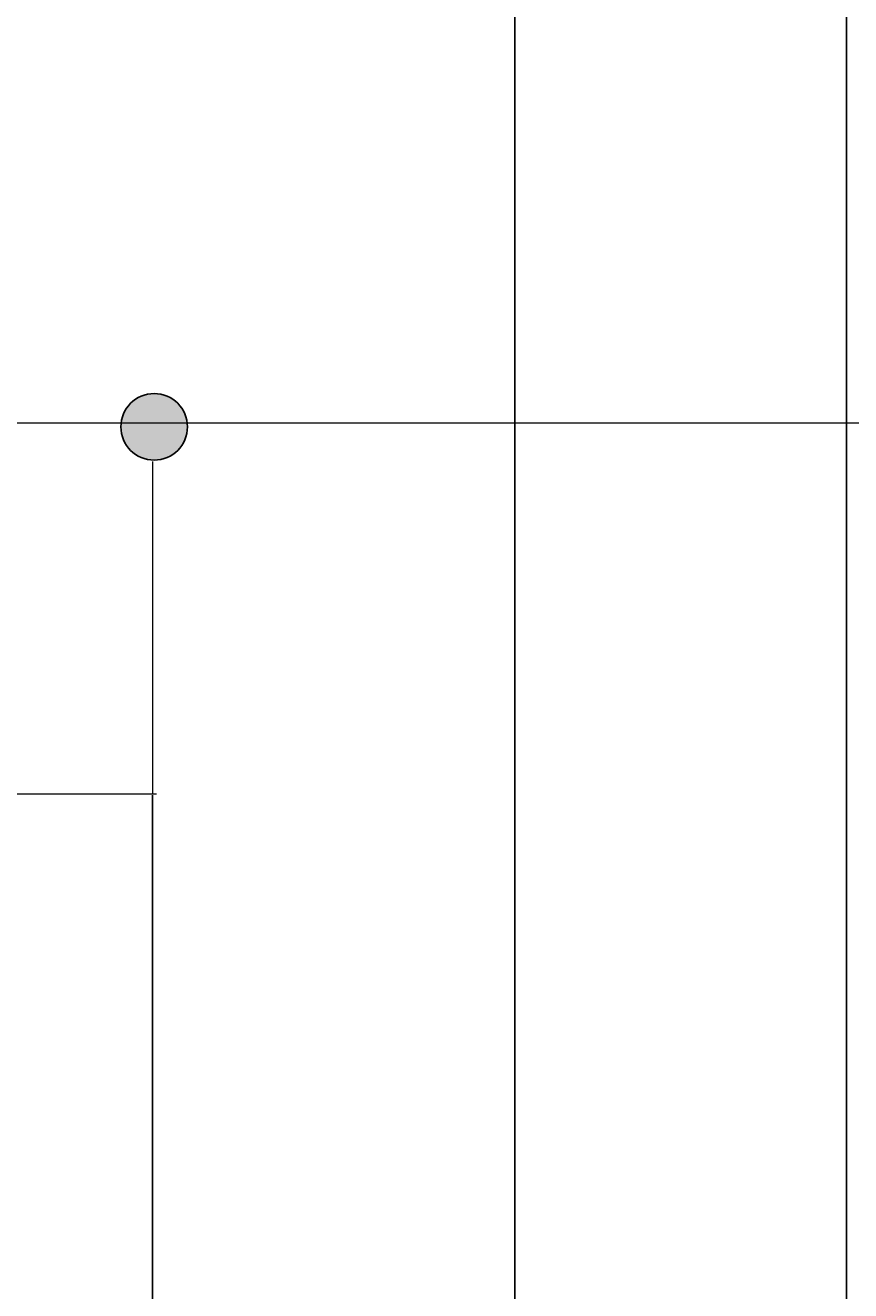
# Model space of a CAD drawing. Units: inches. Extents: x 738 to 1068, y 378 to 757.
# Tile 29 of 41: x 901 to 939, y 492 to 549. Entities that reach past the tile are written whole.
import ezdxf

# ---------------------------------------------------------------- set-up
doc = ezdxf.new("R2010")
doc.units = ezdxf.units.IN
doc.header["$MEASUREMENT"] = 0
for name, color, linetype, lineweight in [('A-ANNO-DIMS', 2, 'Continuous', 18), ('E-CONN', 7, 'Continuous', 25), ('E-CONN-PATT', 7, 'Continuous', 13), ('E-CTRL-WIRE', 7, 'Continuous', 18)]:
    doc.layers.add(name, color=color, linetype=linetype, lineweight=lineweight)
doc.styles.get("Standard").update_dxf_attribs({"font": 'arial.ttf'})
doc.dimstyles.get("Standard").update_dxf_attribs({"dimtxt": 0.18, "dimasz": 0.18, "dimexe": 0.18, "dimexo": 0.0625, "dimgap": 0.09, "dimtad": 0, "dimtih": 1, "dimtoh": 1, "dimdec": 4, "dimzin": 0, "dimdsep": 46, "dimtxsty": 'Standard', "dimcen": 0.09, "dimadec": 0, "dimazin": 0, "dimtfac": 1, "dimtdec": 4, "dimtofl": 0, "dimtmove": 0, "dimatfit": 3, "dimfxl": 1, "dimtolj": 1, "dimtzin": 0, "dimarcsym": 0})

# ---------------------------------------------------------------- blocks, each defined once
blk = doc.blocks.new('*D18')
at = {"layer": 'A-ANNO-DIMS', "color": 0, "lineweight": -2, "transparency": 16777216}
for p, q in [((901.525, 738.375), (1068.179, 738.375)), ((1067.999, 738.195), (1067.999, 569.167)), ((1067.999, 399.775), (1067.999, 568.803)), ((1023.842, 399.595), (1068.179, 399.595))]:
    blk.add_line(p, q, dxfattribs=at)
at = {"layer": 'A-ANNO-DIMS', "color": 0, "transparency": 16777216}
for points in [[(1067.969, 738.195), (1068.029, 738.195), (1067.999, 738.375)], [(1067.969, 399.775), (1068.029, 399.775), (1067.999, 399.595)]]:
    blk.add_solid(points, dxfattribs=at)
at = {"layer": 'Defpoints', "color": 0, "transparency": 16777216}
for p in [(901.462, 738.375), (1067.999, 738.375), (1023.779, 399.595)]:
    blk.add_point(p, dxfattribs=at)
at = {"layer": 'A-ANNO-DIMS', "color": 0, "transparency": 16777216, "insert": (1067.999, 568.985), "char_height": 0.18, "attachment_point": 5}
blk.add_mtext('\\A1;338.8', dxfattribs=at)
blk = doc.blocks.new('*D27')
at = {"layer": 'A-ANNO-DIMS', "color": 0, "lineweight": -2, "transparency": 16777216}
for p, q in [((883.457, 646.923), (883.457, 378.239)), ((923.511, 646.923), (923.511, 378.239)), ((883.637, 378.419), (903.086, 378.419)), ((923.331, 378.419), (903.882, 378.419))]:
    blk.add_line(p, q, dxfattribs=at)
at = {"layer": 'A-ANNO-DIMS', "color": 0, "transparency": 16777216}
for points in [[(883.637, 378.449), (883.637, 378.389), (883.457, 378.419)], [(923.331, 378.449), (923.331, 378.389), (923.511, 378.419)]]:
    blk.add_solid(points, dxfattribs=at)
at = {"layer": 'Defpoints', "color": 0, "transparency": 16777216}
for p in [(883.457, 646.985), (923.511, 646.985), (923.511, 378.419)]:
    blk.add_point(p, dxfattribs=at)
at = {"layer": 'A-ANNO-DIMS', "color": 0, "transparency": 16777216, "insert": (903.484, 378.419), "char_height": 0.18, "attachment_point": 5}
blk.add_mtext('\\A1;40.05', dxfattribs=at)
blk = doc.blocks.new('*D28')
at = {"layer": 'A-ANNO-DIMS', "color": 0, "lineweight": -2, "transparency": 16777216}
for p, q in [((923.511, 646.923), (923.511, 378.239)), ((969.439, 646.923), (969.439, 378.239)), ((923.691, 378.419), (946.078, 378.419)), ((969.259, 378.419), (946.872, 378.419))]:
    blk.add_line(p, q, dxfattribs=at)
at = {"layer": 'A-ANNO-DIMS', "color": 0, "transparency": 16777216}
for points in [[(923.691, 378.449), (923.691, 378.389), (923.511, 378.419)], [(969.259, 378.449), (969.259, 378.389), (969.439, 378.419)]]:
    blk.add_solid(points, dxfattribs=at)
at = {"layer": 'Defpoints', "color": 0, "transparency": 16777216}
for p in [(923.511, 646.985), (969.439, 646.985), (969.439, 378.419)]:
    blk.add_point(p, dxfattribs=at)
at = {"layer": 'A-ANNO-DIMS', "color": 0, "transparency": 16777216, "insert": (946.475, 378.419), "char_height": 0.18, "attachment_point": 5}
blk.add_mtext('\\A1;45.93', dxfattribs=at)
blk = doc.blocks.new('*D33')
at = {"layer": 'A-ANNO-DIMS', "color": 0, "lineweight": -2, "transparency": 16777216}
for p, q in [((836.324, 514.624), (836.324, 378.239)), ((907.171, 514.624), (907.171, 378.239)), ((836.504, 378.419), (871.354, 378.419)), ((906.991, 378.419), (872.141, 378.419))]:
    blk.add_line(p, q, dxfattribs=at)
at = {"layer": 'A-ANNO-DIMS', "color": 0, "transparency": 16777216}
for points in [[(836.504, 378.449), (836.504, 378.389), (836.324, 378.419)], [(906.991, 378.449), (906.991, 378.389), (907.171, 378.419)]]:
    blk.add_solid(points, dxfattribs=at)
at = {"layer": 'Defpoints', "color": 0, "transparency": 16777216}
for p in [(836.324, 514.687), (907.171, 514.687), (907.171, 378.419)]:
    blk.add_point(p, dxfattribs=at)
at = {"layer": 'A-ANNO-DIMS', "color": 0, "transparency": 16777216, "insert": (871.748, 378.419), "char_height": 0.18, "attachment_point": 5}
blk.add_mtext('\\A1;70.85', dxfattribs=at)
blk = doc.blocks.new('*D39')
at = {"layer": 'A-ANNO-DIMS', "color": 0, "lineweight": -2, "transparency": 16777216}
for p, q in [((887.04, 581.418), (887.04, 378.239)), ((938.455, 581.418), (938.455, 378.239)), ((887.22, 378.419), (912.371, 378.419)), ((938.275, 378.419), (913.124, 378.419))]:
    blk.add_line(p, q, dxfattribs=at)
at = {"layer": 'A-ANNO-DIMS', "color": 0, "transparency": 16777216}
for points in [[(887.22, 378.449), (887.22, 378.389), (887.04, 378.419)], [(938.275, 378.449), (938.275, 378.389), (938.455, 378.419)]]:
    blk.add_solid(points, dxfattribs=at)
at = {"layer": 'Defpoints', "color": 0, "transparency": 16777216}
for p in [(887.04, 581.481), (938.455, 581.481), (938.455, 378.419)]:
    blk.add_point(p, dxfattribs=at)
at = {"layer": 'A-ANNO-DIMS', "color": 0, "transparency": 16777216, "insert": (912.748, 378.419), "char_height": 0.18, "attachment_point": 5}
blk.add_mtext('\\A1;51.41', dxfattribs=at)

msp = doc.modelspace()

# ---------------------------------------------------------------- hatches: boundary and pattern name
at = {"layer": 'E-CONN-PATT'}
h = msp.add_hatch(color=256, dxfattribs=at)
h.dxf.hatch_style = 1
h.paths.add_polyline_path([(834.743, 531.4009), (837.7218, 531.4009, 0.8876841)])
h.paths.add_polyline_path([(837.7324, 531.2231, 0.0297234), (837.7218, 531.4009), (834.743, 531.4009, 0.0297234), (834.7324, 531.2231, 1)])
h.paths.add_polyline_path([(908.7522, 531.2231, 0.0297234), (908.7416, 531.4009), (905.7628, 531.4009, 0.0297234), (905.7522, 531.2231, 1)])
h.paths.add_polyline_path([(905.7628, 531.4009), (908.7416, 531.4009, 0.8876841)])

# ---------------------------------------------------------------- linework, layer by layer
at = {"layer": 'E-CONN'}
msp.add_lwpolyline([(905.7522, 531.2231, 1), (908.7522, 531.2231, 1)], format="xyb", close=True, dxfattribs=at)
at = {"layer": 'E-CTRL-WIRE'}
for p, q in [((885.9574, 531.4009), (966.9395, 531.4009)), ((907.1708, 529.6579), (907.1708, 514.6866)), ((877.3586, 514.6866), (907.3586, 514.6866))]:
    msp.add_line(p, q, dxfattribs=at)

# ---------------------------------------------------------------- dimensions: what is measured, and where the dimension line sits
at = {"layer": 'A-ANNO-DIMS'}
dim = msp.add_linear_dim(base=(1067.9992, 738.3751), p1=(1023.779, 399.5952), p2=(901.4622, 738.3751), angle=90, dimstyle='Standard', override={"dimdec": 1, "dimlfac": 1, "dimrnd": 0, "dimzin": 0, "dimdsep": 46, "dimlunit": 2}, dxfattribs=at)
dim.commit()
dim.dimension.update_dxf_attribs({"geometry": '*D18', "text_midpoint": (1067.9992, 568.9851)})
for base, p1, p2, picture, middle in [((923.5105, 378.4191), (883.4574, 646.9853), (923.5105, 646.9853), '*D27', (903.484, 378.4191)), ((969.4395, 378.4191), (923.5105, 646.9853), (969.4395, 646.9853), '*D28', (946.475, 378.4191)), ((938.455, 378.4191), (887.0404, 581.4808), (938.455, 581.4808), '*D39', (912.7477, 378.4191)), ((907.1708, 378.4191), (836.3244, 514.6866), (907.1708, 514.6866), '*D33', (871.7476, 378.4191))]:
    dim = msp.add_linear_dim(base=base, p1=p1, p2=p2, dimstyle='Standard', override={"dimdec": 2, "dimlfac": 1, "dimrnd": 0, "dimzin": 0, "dimdsep": 46, "dimlunit": 2}, dxfattribs=at)
    dim.commit()
    dim.dimension.update_dxf_attribs({"geometry": picture, "text_midpoint": middle})

doc.saveas('drawing.dxf')
